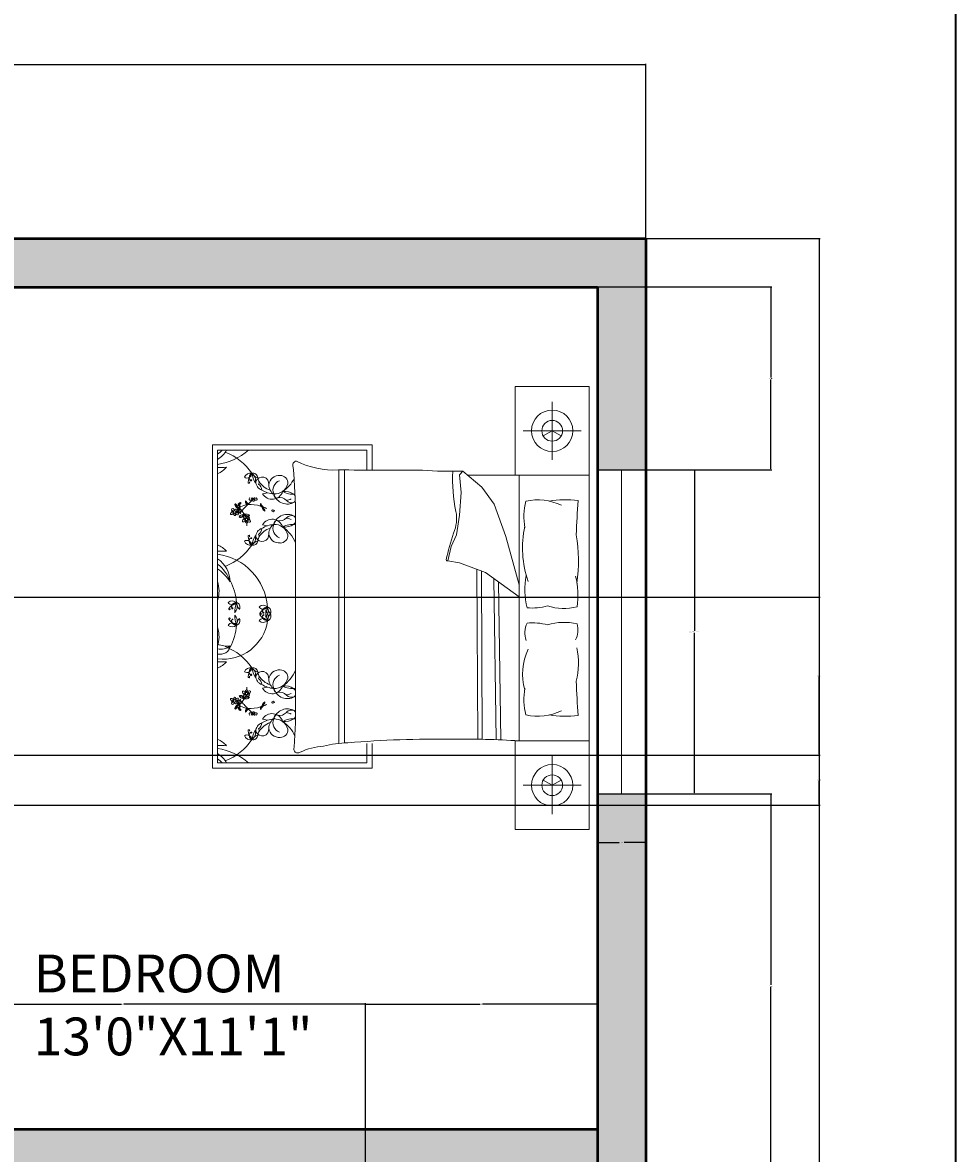
# Model space of a CAD drawing. Units: inches. Extents: x 1676 to 2199, y 1657 to 2783.
# Tile 9 of 10: x 2027 to 2199, y 2172 to 2381. Entities that reach past the tile are written whole.
import ezdxf

# ---------------------------------------------------------------- set-up
doc = ezdxf.new("R2010")
doc.units = ezdxf.units.IN
for name, color, linetype, lineweight in [('A-ANNO-DIMS', 2, 'Continuous', 18), ('A-ANNO-TTLB', 7, 'Continuous', 35), ('A-AREA-IDEN', 7, 'Continuous', 18), ('A-FURN', 8, 'Continuous', 13), ('A-GLAZ', 4, 'Continuous', 18), ('A-WALL', 7, 'Continuous', 50)]:
    doc.layers.add(name, color=color, linetype=linetype, lineweight=lineweight)
doc.layers.add('A-WALL-PATT', color=251, linetype='Continuous', lineweight=13, true_color=0x636466)
doc.styles.get("Standard").update_dxf_attribs({"font": 'arial.ttf'})
doc.dimstyles.get("Standard").update_dxf_attribs({"dimtxt": 0.18, "dimasz": 0.18, "dimexe": 0.18, "dimexo": 0.0625, "dimgap": 0.09, "dimtad": 0, "dimtih": 1, "dimtoh": 1, "dimdec": 4, "dimzin": 0, "dimdsep": 46, "dimtxsty": 'Standard', "dimcen": 0.09, "dimadec": 0, "dimazin": 0, "dimtfac": 1, "dimtdec": 4, "dimtofl": 0, "dimtmove": 0, "dimatfit": 3, "dimfxl": 1, "dimtolj": 1, "dimtzin": 0, "dimarcsym": 0})

# ---------------------------------------------------------------- blocks, each defined once
blk = doc.blocks.new('BED-DOUBLE-WITH-NIGHTSTANDS')
for p, q in [((0, 0), (0, -82.08)), ((-6.84, -13.57), (-6.84, -2.85)), ((-12.2, -8.21), (-1.48, -8.21)), ((-69.81, -10.83), (-40.24, -10.83)), ((-69.81, -70.68), (-69.81, -10.83)), ((-68.85, -11.79), (-68.85, -69.72)), ((-41.19, -11.79), (-68.85, -11.79)), ((-41.19, -15.48), (-41.19, -11.79)), ((-40.24, -10.83), (-40.24, -15.48)), ((-46.38, -66.12), (-46.38, -15.47)), ((-45.36, -66.04), (-45.36, -15.47)), ((-24.05, -16.35), (-23.39, -15.68)), ((-23.72, -19.67), (-24.05, -16.35)), ((-23.39, -15.68), (-19.9, -18.67)), ((0, -16.42), (-22.53, -16.42)), ((-12.97, -16.42), (-12.97, -65.67)), ((-19.9, -18.67), (-17.57, -21.83)), ((-60.53, -19.87), (-59.61, -19.69)), ((-24.05, -23.83), (-23.72, -19.67)), ((-17.57, -21.83), (-15.41, -27.82)), ((-54.44, -57.71), (-54.44, -24.38)), ((-24.55, -27.49), (-24.05, -23.83)), ((-60.53, -25.61), (-59.61, -25.79)), ((-25.55, -29.65), (-24.55, -27.49)), ((-15.41, -27.82), (-12.97, -36.77)), ((-26.21, -32.31), (-25.55, -29.65)), ((-24.05, -32.64), (-26.21, -32.31)), ((-19.23, -34.47), (-24.05, -32.64)), ((-20.65, -65.38), (-20.78, -33.88)), ((-19.81, -65.37), (-19.93, -34.2)), ((-12.97, -38.97), (-19.23, -34.47)), ((-17.22, -65.41), (-17.64, -35.61)), ((-16.38, -65.45), (-16.79, -36.22)), ((-60.53, -55.9), (-59.61, -55.72)), ((-60.53, -61.64), (-59.61, -61.82)), ((-41.19, -69.72), (-41.19, -66.11)), ((-40.24, -66.12), (-40.24, -70.68)), ((-6.84, -68.51), (-6.84, -79.24)), ((-40.24, -70.68), (-69.81, -70.68)), ((-68.85, -69.72), (-41.19, -69.72)), ((-12.2, -73.87), (-1.48, -73.87))]:
    blk.add_line(p, q)
for points in [[(-13.68, -16.42), (-13.68, 0), (0, 0)], [(-6.84, -8.21), (-8.5, -9.17)], [(-6.84, -8.21), (-5.18, -9.17)], [(0, -65.67), (-13.68, -65.67), (-13.68, -82.08), (0, -82.08)], [(-6.84, -73.87), (-8.5, -72.92)], [(-6.84, -73.87), (-5.18, -72.92)]]:
    blk.add_lwpolyline(points)
for points in [[(-30.9, -15.51, 0.001242), (-46.48, -15.47, -0.127202), (-54.24, -13.83)], [(-2.05, -21.13, 0.074897), (-7.41, -21.23, -0.472817)], [(-7.71, -40.66, 0.14099), (-2.24, -40.82, 0.235245)], [(-7.71, -44.16, -0.14099), (-2.24, -44, -0.235245)], [(-2.05, -60.95, -0.074897), (-7.41, -60.85, 0.472817)], [(-44.71, -66.02, 0.056112), (-49.23, -66.61, 0.095341), (-53.58, -67.77)]]:
    blk.add_lwpolyline(points, format="xyb")
for centre, radius in [((-6.84, -8.21), 3.83), ((-6.84, -8.21), 1.92), ((-65.71, -23.25), 0.209), ((-63.51, -24.62), 0.209), ((-65.71, -58.26), 0.209), ((-63.51, -56.89), 0.209), ((-6.84, -73.87), 3.83), ((-6.84, -73.87), 1.92)]:
    blk.add_circle(centre, radius)
for centre, radius, start, end in [((-72.71, -7.3), 6.51, 306.3036, 316.4814), ((-71.73, -9.18), 5.22, 303.4617, 330.1116), ((-70.3, -3.81), 10.72, 277.745, 311.8856), ((-71.36, -22.14), 10.72, 34.3865, 68.5908), ((-54.19, -14.58), 0.757, 93.98, 207.3412), ((-70.53, -12.11), 4.36, 292.5547, 318.9546), ((-68.18, -0.17), 14.83, 267.4081, 273.6519), ((-62.77, -17.25), 1.19, 77.7115, 159.0387), ((-63.41, -16.06), 0.895, 238.4633, 358.2869), ((-60.47, -17.87), 2.71, 138.8402, 177.9352), ((-62.11, -16.87), 0.877, 117.6827, 223.7762), ((-62.3, -16.95), 0.889, 2.9516, 103.728), ((-55.19, -14.46), 7.5, 192.5173, 207.1824), ((-63.5, -17.46), 1.69, 345.4653, 54.2343), ((-60.95, -15.14), 1.83, 211.3827, 255.2969), ((-57.44, -18.45), 1.96, 84.9449, 172.8857), ((-57.24, -17.88), 1.39, 354.4856, 91.0538), ((-139.89, -23.4), 85.45, 359.3433, 5.6887), ((-25.43, 59.58), 75.29, 265.8294, 271.553), ((5.68, -17.09), 30.98, 177.4519, 191.3392), ((-63.05, -17.78), 0.133, 177.9352, 11.4834), ((-62.98, -17.77), 0.0647, 11.4834, 127.9409), ((-62.66, -17.39), 0.116, 223.7762, 159.7183), ((-60.23, -17.7), 1.54, 175.969, 254.3045), ((-60.6, -18), 1.23, 350.264, 160.8688), ((-61.93, -17.74), 0.755, 333.9755, 53.2681), ((-62.27, -19.36), 1.64, 6.1662, 51.5825), ((-57.89, -15.55), 3.88, 211.2614, 251.7045), ((-57, -18.11), 2.38, 182.3591, 234.0401), ((-56.7, -19.22), 1.9, 111.5819, 201.4221), ((-58.27, -17.45), 2.47, 265.2933, 346.921), ((-60.22, -14.26), 6.21, 303.6671, 333.2997), ((-62.86, -20.88), 0.16, 142.4737, 265.053), ((-62.65, -20.85), 0.345, 127.7621, 169.0403), ((-62.84, -20.56), 0.486, 265.053, 338.3618), ((-62.19, -21.22), 0.635, 113.4276, 137.6104), ((-62.27, -20.56), 0.209, 183.2768, 356.7232), ((-62.11, -20.94), 0.342, 139.7889, 227.6792), ((-62.92, -20.94), 0.684, 353.0852, 15.7171), ((-62.47, -21.02), 0.432, 350.3487, 43.6538), ((-61.67, -20.57), 0.503, 198.7263, 262.5032), ((-62.07, -20.81), 0.2, 1.1081, 91.8675), ((-61.94, -20.85), 0.349, 11.5637, 52.6358), ((-61.69, -20.92), 0.162, 255.2356, 54.9248), ((-58.2, -15.52), 4.4, 236.2883, 266.5076), ((-58.76, -18.86), 2.04, 209.9085, 343.1337), ((-57.91, -20.15), 0.509, 167.3041, 285.1471), ((-56.53, -22.59), 3.17, 122.7011, 126.3445), ((-55.93, -19.17), 2.62, 199.2822, 299.1751), ((-57.33, -22.26), 1.68, 41.5653, 105.1471), ((-55.05, -16.54), 3.4, 238.8218, 279.1554), ((-56.53, -22.59), 3.17, 55.785, 94.7304), ((-56.41, -18.78), 2.36, 277.436, 299.9149), ((-55.35, -20.75), 0.989, 30.0293, 52.325), ((-65.87, -22.82), 0.413, 157.4086, 261.4386), ((-66.1, -22.81), 0.207, 58.0499, 135.6268), ((-65.89, -22.94), 0.138, 172.906, 277.132), ((-66.34, -23.19), 0.659, 14.7558, 58.0499), ((-65.42, -23.02), 0.285, 36.1046, 181.4281), ((-65.41, -21.9), 0.233, 124.3538, 214.3923), ((-65.06, -21.94), 0.544, 190.3057, 287.1958), ((-65.59, -22.79), 0.288, 270.0645, 331.1507), ((-64.91, -21.74), 0.632, 176.9701, 248.2913), ((-60.4, -18.41), 6.11, 212.6784, 216.3746), ((-65.34, -22.99), 0.205, 263.7526, 41.7054), ((-65.12, -21.89), 0.242, 216.3746, 291.7548), ((-62.98, -25.28), 3.41, 124.0033, 132.4917), ((-66.49, -25.71), 3.64, 63.7819, 68.2913), ((-64.54, -22.91), 0.579, 128.3208, 208.8162), ((-64.54, -22.06), 0.544, 122.8155, 187.3992), ((-64.96, -22.28), 0.182, 289.3605, 111.7548), ((-64.83, -22.28), 0.182, 221.8703, 44.2646), ((-64, -22.81), 0.953, 157.2305, 229.0635), ((-64.3, -22.13), 0.632, 109.4799, 177.6828), ((-64.32, -22.5), 0.561, 174.4544, 220.6188), ((-67.51, -25.63), 4.09, 30.544, 49.818), ((-64.64, -21.73), 0.233, 56.8636, 146.9021), ((-64.52, -21.99), 0.242, 148.8844, 224.2646), ((-65.26, -23.3), 0.674, 340.0041, 40.6188), ((-59.5, -25.02), 6.11, 145.1882, 148.8844), ((-62.98, -25.28), 3.41, 94.756, 119.2041), ((-55.72, -30.19), 11.22, 132.2412, 142.1744), ((-61.39, -21.26), 2.31, 178.3264, 187.1302), ((-63.89, -21.58), 0.431, 11.3256, 64.4621), ((-62.42, -20.96), 1.3, 190.2588, 210.656), ((-63.29, -21.49), 0.394, 188.3432, 274.2869), ((-62.95, -21.27), 0.688, 210.656, 242.6341), ((-62.43, -20.68), 1.32, 218.2101, 226.3071), ((-63.4, -21.79), 0.167, 325.7657, 67.4417), ((-68.6, -16.2), 7.79, 313.1541, 322.0459), ((-62.81, -28.67), 6.8, 73.5842, 93.8277), ((-62.22, -21.06), 0.18, 227.6792, 350.3487), ((-58.62, -21.75), 2.31, 178.3264, 187.1302), ((-61.12, -22.07), 0.431, 11.3256, 64.4621), ((-59.66, -21.45), 1.3, 190.2588, 210.656), ((-60.53, -21.98), 0.394, 188.3432, 274.2869), ((-60.19, -21.76), 0.688, 210.656, 242.6341), ((-59.67, -21.17), 1.32, 218.2101, 226.3071), ((-60.64, -22.28), 0.167, 325.7657, 67.4417), ((-60.17, -22.58), 0.394, 147.5332, 233.4768), ((-59.81, -22.38), 0.688, 179.1859, 211.164), ((-60.49, -22.54), 0.167, 354.3784, 96.0543), ((-62.81, -28.67), 6.8, 63.0032, 69.8941), ((-59.29, -22.07), 1.3, 211.164, 231.5612), ((-59.07, -21.01), 2.31, 234.6898, 243.4936), ((-59.05, -22.2), 1.32, 195.5129, 203.6099), ((-60.53, -23.06), 0.431, 357.3579, 50.4944), ((-58.68, -22.98), 0.158, 12.7051, 190.4384), ((-58.58, -22.96), 0.257, 190.4384, 10.4136), ((-55.16, -20.33), 1.23, 221.5653, 293.8354), ((-55.35, -20.75), 0.989, 314.4517, 333.558), ((-1.09, -24.06), 11, 165.1039, 191.0369), ((-9.56, -31.59), 10.58, 65.1316, 101.7583), ((779.11, -66.37), 782.47, 176.68521, 177.14978), ((-66.31, -23.57), 0.16, 142.4737, 265.053), ((-66.1, -23.53), 0.345, 61.2196, 169.0403), ((-66.28, -23.24), 0.486, 265.053, 338.3618), ((-65.64, -23.91), 0.635, 113.4276, 137.6104), ((-65.56, -23.63), 0.342, 139.7889, 227.6792), ((-65.67, -23.75), 0.18, 227.6792, 350.3487), ((-66.36, -23.62), 0.684, 353.0852, 15.7171), ((-65.91, -23.7), 0.432, 350.3487, 43.6538), ((-65.34, -22.86), 0.329, 221.8413, 265.7877), ((-65.11, -23.26), 0.503, 198.7263, 262.5032), ((-65.51, -23.49), 0.2, 1.1081, 91.8675), ((-65.39, -23.54), 0.349, 11.5637, 86.365), ((-65.14, -23.6), 0.162, 255.2356, 54.9248), ((-64.44, -22.87), 0.692, 207.7043, 254.3516), ((-64.89, -23.26), 0.953, 270.278, 342.111), ((-64.25, -24.45), 0.674, 98.7227, 159.3375), ((-64.59, -23.59), 0.692, 244.9899, 291.6373), ((-64.44, -23.23), 0.561, 278.7227, 324.8872), ((-64.54, -23.69), 0.579, 290.5253, 358.5375), ((-64.11, -24.93), 0.16, 142.4737, 265.053), ((-63.89, -24.9), 0.345, 61.2196, 169.0403), ((-64.08, -24.61), 0.486, 265.053, 338.3618), ((-63.67, -24.19), 0.413, 157.4086, 261.4386), ((-63.9, -24.18), 0.207, 58.0499, 135.6268), ((-63.41, -23.52), 0.579, 182.8499, 266.1226), ((-63.63, -23.12), 0.561, 231.7607, 277.9252), ((-63.2, -23.02), 0.953, 214.5369, 286.3699), ((-63.43, -25.27), 0.635, 113.4276, 137.6104), ((-63.68, -24.31), 0.138, 172.906, 277.132), ((-64.14, -24.56), 0.659, 14.7558, 58.0499), ((-67.51, -25.63), 4.09, 23.0501, 23.8477), ((-63.35, -24.99), 0.342, 139.7889, 227.6792), ((-63.46, -24.34), 0.674, 37.3105, 97.9252), ((-63.22, -24.39), 0.285, 36.1046, 181.4281), ((-64.16, -24.99), 0.684, 353.0852, 15.7171), ((-63.39, -23.41), 0.692, 265.0106, 311.658), ((-63.71, -25.07), 0.432, 350.3487, 43.6538), ((-62.91, -24.63), 0.503, 198.7263, 262.5032), ((-63.38, -24.16), 0.288, 270.0645, 331.1507), ((-63.14, -24.23), 0.329, 221.8413, 265.7877), ((-63.31, -24.86), 0.2, 1.1081, 91.8675), ((-63.14, -24.35), 0.205, 263.7526, 41.7054), ((-63.18, -24.91), 0.349, 11.5637, 86.365), ((-62.93, -24.97), 0.162, 255.2356, 54.9248), ((-58.76, -26.63), 2.04, 16.8663, 150.0915), ((-57.91, -25.34), 0.509, 74.8529, 192.6959), ((-55.93, -26.31), 2.62, 60.8249, 160.7178), ((-57.33, -23.22), 1.68, 254.8529, 318.4347), ((-56.41, -26.71), 2.36, 60.0851, 82.564), ((-55.16, -25.15), 1.23, 66.1646, 138.4347), ((-55.35, -24.73), 0.989, 307.675, 336.7144), ((-55.35, -24.73), 0.989, 23.229, 45.5483), ((-31.24, -24.49), 6.68, 336.2616, 11.3392), ((-63.46, -25.11), 0.18, 227.6792, 350.3487), ((-67.51, -25.63), 4.09, 357.1071, 4.7585), ((-60.23, -27.78), 1.54, 105.6955, 184.031), ((-62.27, -26.13), 1.64, 308.4175, 353.8338), ((-57.89, -29.93), 3.88, 108.2955, 148.7386), ((-58.2, -29.97), 4.4, 93.4924, 123.7117), ((-57, -27.38), 2.38, 125.9599, 177.6409), ((-56.7, -26.27), 1.9, 158.5779, 248.4181), ((-58.27, -28.03), 2.47, 13.079, 94.7067), ((-56.53, -22.9), 3.17, 233.6555, 237.2989), ((-55.05, -28.95), 3.4, 79.7133, 121.1782), ((-56.53, -22.9), 3.17, 265.2696, 304.215), ((-60.22, -31.22), 6.21, 21.4941, 56.3329), ((4.81, -38.01), 31.83, 160.1194, 169.3383), ((6.73, -29.85), 19.08, 168.0397, 199.2615), ((-63.41, -29.42), 0.895, 1.7131, 121.5367), ((-62.77, -28.23), 1.19, 200.9613, 282.2885), ((-63.05, -27.7), 0.133, 348.5166, 182.0648), ((-60.47, -27.61), 2.71, 182.0648, 221.1598), ((-62.98, -27.72), 0.0647, 232.0591, 348.5166), ((-62.11, -28.62), 0.877, 136.2238, 242.3173), ((-62.61, -28.1), 0.0699, 200.2667, 136.2271), ((-63.5, -28.02), 1.69, 305.7657, 14.5347), ((-55.19, -31.02), 7.5, 152.8176, 167.4827), ((-62.3, -28.53), 0.889, 256.272, 357.0484), ((-60.95, -30.35), 1.83, 104.7031, 148.6173), ((-60.6, -27.49), 1.23, 199.1312, 9.736), ((-61.93, -27.74), 0.755, 306.7319, 26.0245), ((-57.44, -27.04), 1.96, 187.1143, 275.0551), ((-57.24, -27.61), 1.39, 268.9462, 5.5144), ((-31.75, -32.38), 29.77, 352.2196, 9.497), ((-70.53, -33.38), 4.36, 41.0454, 67.4453), ((-68.18, -45.32), 14.83, 86.3481, 92.5919), ((-70.3, -41.68), 10.72, 4.4623, 82.255), ((-71.36, -23.34), 10.72, 291.4092, 325.6135), ((-71.73, -36.3), 5.22, 1.272, 56.5383), ((-72.71, -38.18), 6.51, 17.8504, 53.6964), ((-26.28, -32.12), 0.198, 178.8623, 289.7536), ((-74.54, -41.6), 9.68, 34.0123, 54.053), ((2.57, -37.57), 14.48, 169.8617, 193.6238), ((-16.7, -38.67), 14.63, 351.5249, 13.96), ((-74.49, -37.86), 5.89, 343.5431, 17.0202), ((-76.04, -40.86), 10.72, 4.4623, 27.4146), ((-77.53, -40.2), 8.72, 4.3787, 5.6357), ((-83.5, -44.79), 15.58, 19.7217, 19.9028), ((-66.15, -40.91), 1.19, 47.7873, 129.1145), ((-66.12, -39.56), 0.895, 208.5391, 328.3627), ((-66.66, -41.22), 0.133, 148.011, 341.5592), ((-64.48, -42.59), 2.71, 108.9159, 148.011), ((-66.6, -41.25), 0.0647, 341.5592, 98.0167), ((-65.39, -40.9), 0.877, 87.7585, 193.852), ((-66.13, -41.08), 0.116, 193.852, 129.9245), ((-58.2, -42.27), 7.5, 162.593, 177.2582), ((-66.9, -40.72), 1.69, 315.5411, 24.3101), ((-63.52, -39.98), 1.83, 181.4585, 225.3727), ((-65.6, -40.88), 0.889, 333.0274, 73.8037), ((-60.41, -41.73), 1.19, 47.7873, 129.1145), ((-60.38, -40.38), 0.895, 208.5391, 328.3627), ((-58.73, -43.41), 2.71, 108.9159, 148.011), ((-59.65, -41.72), 0.877, 87.7585, 193.852), ((-60.39, -41.9), 0.116, 193.852, 129.9245), ((-61.16, -41.54), 1.69, 315.5411, 24.3101), ((-52.46, -43.09), 7.5, 162.593, 177.2582), ((-61.16, -42.7), 1.69, 335.6899, 44.4589), ((-52.46, -41.16), 7.5, 182.7418, 197.407), ((-59.86, -41.7), 0.889, 333.0274, 73.8037), ((-57.78, -40.8), 1.83, 181.4585, 225.3727), ((-10.45, -30.98), 10.06, 264.0129, 285.8293), ((-67.82, -42.22), 8.3, 262.8636, 351.8197), ((-66.12, -44.69), 0.895, 31.6373, 151.4609), ((-66.66, -43.02), 0.133, 18.4408, 211.989), ((-64.48, -41.66), 2.71, 211.989, 251.0841), ((-66.6, -43), 0.0647, 261.9833, 18.4408), ((-65.39, -43.35), 0.877, 166.148, 272.2415), ((-66.08, -43.15), 0.0699, 230.1909, 166.0209), ((-58.2, -41.98), 7.5, 182.7418, 197.407), ((-66.9, -43.52), 1.69, 335.6899, 44.4589), ((-63.52, -44.27), 1.83, 134.6273, 178.5415), ((-65.6, -43.37), 0.889, 286.1963, 26.9726), ((-60.38, -43.87), 0.895, 31.6373, 151.4609), ((-60.41, -42.52), 1.19, 230.8855, 312.2127), ((-60.92, -42.04), 0.133, 148.011, 341.5592), ((-60.92, -42.2), 0.133, 18.4408, 211.989), ((-58.73, -40.84), 2.71, 211.989, 251.0841), ((-60.86, -42.07), 0.0647, 341.5592, 98.0167), ((-60.86, -42.18), 0.0647, 261.9833, 18.4408), ((-59.65, -42.52), 0.877, 166.148, 272.2415), ((-60.34, -42.33), 0.0699, 230.1909, 166.0209), ((-59.86, -42.55), 0.889, 286.1963, 26.9726), ((-57.78, -43.45), 1.83, 134.6273, 178.5415), ((-7.56, -45.67), 4.35, 155.0183, 198.5407), ((-10.45, -53.84), 10.06, 74.1707, 95.9871), ((-74.49, -46.39), 5.89, 342.9798, 16.4569), ((-77.53, -44.05), 8.72, 354.3643, 355.6213), ((-83.5, -39.46), 15.58, 340.0972, 340.2783), ((-66.15, -43.34), 1.19, 230.8855, 312.2127), ((-76.04, -43.39), 10.72, 332.5854, 355.5377), ((-6.14, -45.12), 4.06, 333.3437, 16.1026), ((-67.07, -43.29), 4.8, 248.117, 276.6195), ((-68.4, -47.7), 1.92, 256.3898, 349.0739), ((-68.14, -46.25), 2.43, 252.8609, 311.9049), ((-71.36, -58.17), 10.72, 34.3865, 68.5908), ((-1.9, -53.28), 10.45, 153.8761, 196.1746), ((-16.41, -51.21), 14.43, 346.3427, 11.1841), ((-68.18, -36.19), 14.83, 267.4081, 273.6519), ((-70.53, -48.13), 4.36, 292.5547, 318.9546), ((-62.77, -53.28), 1.19, 77.7115, 159.0387), ((-63.41, -52.09), 0.895, 238.4633, 358.2869), ((-60.47, -53.9), 2.71, 138.8402, 177.9352), ((-62.11, -52.89), 0.877, 117.6827, 223.7762), ((-62.3, -52.98), 0.889, 2.9516, 103.728), ((-60.95, -51.16), 1.83, 211.3827, 255.2969), ((-63.5, -53.49), 1.69, 345.4653, 54.2343), ((-55.19, -50.49), 7.5, 192.5173, 207.1824), ((-63.05, -53.81), 0.133, 177.9352, 11.4834), ((-62.98, -53.79), 0.0647, 11.4834, 127.9409), ((-62.66, -53.42), 0.116, 223.7762, 159.7183), ((-60.23, -53.73), 1.54, 175.969, 254.3045), ((-60.6, -54.02), 1.23, 350.264, 160.8688), ((-61.93, -53.77), 0.755, 333.9755, 53.2681), ((-62.27, -55.38), 1.64, 6.1662, 51.5825), ((-57.89, -51.58), 3.88, 211.2614, 251.7045), ((-57.44, -54.47), 1.96, 84.9449, 172.8857), ((-57, -54.13), 2.38, 182.3591, 234.0401), ((-56.7, -55.24), 1.9, 111.5819, 201.4221), ((-58.27, -53.48), 2.47, 265.2933, 346.921), ((-57.24, -53.9), 1.39, 354.4856, 91.0538), ((-60.22, -50.29), 6.21, 303.6671, 338.5059), ((-64.11, -56.58), 0.16, 94.947, 217.5263), ((-64.08, -56.9), 0.486, 21.6382, 94.947), ((-63.35, -56.52), 0.342, 132.3208, 220.2111), ((-63.46, -56.4), 0.18, 9.6513, 132.3208), ((-64.16, -56.52), 0.684, 344.2829, 6.9148), ((-67.51, -55.88), 4.09, 355.2415, 2.8929), ((-63.71, -56.44), 0.432, 316.3462, 9.6513), ((-62.91, -56.88), 0.503, 97.4968, 161.2737), ((-62.93, -56.54), 0.162, 305.0752, 104.7644), ((-58.2, -51.54), 4.4, 236.2883, 266.5076), ((-58.76, -54.88), 2.04, 209.9085, 343.1337), ((-57.91, -56.17), 0.509, 167.3041, 285.1471), ((-56.53, -58.61), 3.17, 122.7011, 126.3445), ((-55.93, -55.2), 2.62, 199.2822, 299.1751), ((-55.05, -52.56), 3.4, 238.8218, 280.2867), ((-56.53, -58.61), 3.17, 55.785, 94.7304), ((-55.35, -56.78), 0.989, 23.2856, 52.325), ((-1.09, -58.02), 11, 168.9631, 194.8961), ((779.11, -15.71), 782.47, 182.85022, 183.31479), ((-66.31, -57.94), 0.16, 94.947, 217.5263), ((-66.1, -57.98), 0.345, 190.9597, 298.7804), ((-66.28, -58.27), 0.486, 21.6382, 94.947), ((-65.87, -58.69), 0.413, 98.5614, 202.5914), ((-65.64, -57.6), 0.635, 222.3896, 246.5724), ((-65.89, -58.57), 0.138, 82.868, 187.094), ((-66.34, -58.32), 0.659, 301.9501, 345.2442), ((-65.56, -57.88), 0.342, 132.3208, 220.2111), ((-65.67, -57.76), 0.18, 9.6513, 132.3208), ((-66.36, -57.89), 0.684, 344.2829, 6.9148), ((-65.42, -58.49), 0.285, 178.5719, 323.8954), ((-65.91, -57.81), 0.432, 316.3462, 9.6513), ((-65.11, -58.25), 0.503, 97.4968, 161.2737), ((-65.34, -58.65), 0.329, 94.2123, 138.1587), ((-65.59, -58.72), 0.288, 28.8493, 89.9355), ((-65.51, -58.02), 0.2, 268.1325, 358.8919), ((-65.39, -57.97), 0.349, 273.635, 348.4363), ((-65.34, -58.52), 0.205, 318.2946, 96.2474), ((-65.14, -57.91), 0.162, 305.0752, 104.7644), ((-64.54, -58.6), 0.579, 151.1838, 231.6792), ((-64.44, -58.64), 0.692, 105.6484, 152.2957), ((-64, -58.7), 0.953, 130.9365, 202.7695), ((-64.59, -57.92), 0.692, 68.3627, 115.0101), ((-64.89, -58.25), 0.953, 17.889, 89.722), ((-64.25, -57.06), 0.674, 200.6625, 261.2773), ((-64.32, -59.01), 0.561, 139.3812, 185.5456), ((-67.51, -55.88), 4.09, 310.182, 329.456), ((-65.26, -58.21), 0.674, 319.3812, 19.9959), ((-55.72, -51.32), 11.22, 217.8256, 227.7588), ((-64.44, -58.28), 0.561, 35.1128, 81.2773), ((-64.54, -57.82), 0.579, 1.4625, 69.4747), ((-63.89, -56.61), 0.345, 190.9597, 298.7804), ((-63.67, -57.32), 0.413, 98.5614, 202.5914), ((-63.9, -57.33), 0.207, 224.3732, 301.9501), ((-63.41, -57.99), 0.579, 93.8774, 177.1501), ((-63.2, -58.49), 0.953, 73.6301, 145.4631), ((-63.63, -58.39), 0.561, 82.0748, 128.2393), ((-63.43, -56.24), 0.635, 222.3896, 246.5724), ((-63.68, -57.2), 0.138, 82.868, 187.094), ((-64.14, -56.95), 0.659, 301.9501, 345.2442), ((-67.51, -55.88), 4.09, 336.1523, 336.9499), ((-63.46, -57.17), 0.674, 262.0748, 322.6895), ((-63.22, -57.12), 0.285, 178.5719, 323.8954), ((-63.39, -58.1), 0.692, 48.342, 94.9894), ((-63.14, -57.28), 0.329, 94.2123, 138.1587), ((-63.38, -57.35), 0.288, 28.8493, 89.9355), ((-63.31, -56.65), 0.2, 268.1325, 358.8919), ((-63.18, -56.6), 0.349, 273.635, 348.4363), ((-63.14, -57.16), 0.205, 318.2946, 96.2474), ((-60.17, -58.93), 0.394, 126.5232, 212.4668), ((-59.29, -59.44), 1.3, 128.4388, 148.836), ((-59.07, -60.5), 2.31, 116.5064, 125.3102), ((-60.53, -58.45), 0.431, 309.5056, 2.6421), ((-58.68, -58.53), 0.158, 169.5616, 347.2949), ((-58.58, -58.55), 0.257, 349.5864, 169.5616), ((-57.33, -58.29), 1.68, 41.5653, 105.1471), ((-56.41, -54.8), 2.36, 277.436, 299.9149), ((-55.16, -56.36), 1.23, 221.5653, 293.8354), ((-134.28, -60.22), 79.87, 355.2402, 1.8035), ((-55.35, -56.78), 0.989, 314.4517, 336.7144), ((-66.1, -58.7), 0.207, 224.3732, 301.9501), ((-65.41, -59.61), 0.233, 145.6077, 235.6462), ((-65.06, -59.58), 0.544, 72.8042, 169.6943), ((-64.91, -59.77), 0.632, 111.7087, 183.0299), ((-60.4, -63.1), 6.11, 143.6254, 147.3216), ((-65.12, -59.62), 0.242, 68.2452, 143.6254), ((-62.98, -56.23), 3.41, 227.5083, 235.9967), ((-66.49, -55.8), 3.64, 291.7087, 296.2181), ((-64.54, -59.45), 0.544, 172.6008, 237.1845), ((-64.96, -59.23), 0.182, 248.2452, 70.6395), ((-64.83, -59.23), 0.182, 315.7354, 138.1297), ((-64.3, -59.38), 0.632, 182.3172, 250.5201), ((-64.64, -59.78), 0.233, 213.0979, 303.1364), ((-64.52, -59.52), 0.242, 135.7354, 211.1156), ((-59.5, -56.49), 6.11, 211.1156, 214.8118), ((-62.98, -56.23), 3.41, 240.7959, 265.244), ((-62.42, -60.55), 1.3, 149.344, 169.7412), ((-61.39, -60.25), 2.31, 172.8698, 181.6736), ((-63.89, -59.93), 0.431, 295.5379, 348.6744), ((-63.29, -60.02), 0.394, 85.7131, 171.6568), ((-62.95, -60.24), 0.688, 117.3659, 149.344), ((-62.43, -60.83), 1.32, 133.6929, 141.7899), ((-63.4, -59.72), 0.167, 292.5583, 34.2343), ((-62.81, -52.84), 6.8, 266.1723, 286.4158), ((-68.6, -65.31), 7.79, 37.9541, 46.8459), ((-62.86, -60.63), 0.16, 94.947, 217.5263), ((-62.65, -60.66), 0.345, 190.9597, 232.2379), ((-62.84, -60.95), 0.486, 21.6382, 94.947), ((-62.19, -60.29), 0.635, 222.3896, 246.5724), ((-62.27, -60.95), 0.209, 3.2768, 176.7232), ((-62.11, -60.57), 0.342, 132.3208, 220.2111), ((-62.22, -60.45), 0.18, 9.6513, 132.3208), ((-62.92, -60.57), 0.684, 344.2829, 6.9148), ((-62.47, -60.49), 0.432, 316.3462, 9.6513), ((-61.67, -60.94), 0.503, 97.4968, 161.2737), ((-62.07, -60.7), 0.2, 268.1325, 358.8919), ((-61.69, -60.6), 0.162, 305.0752, 104.7644), ((-61.94, -60.66), 0.349, 307.3642, 348.4363), ((-59.66, -60.06), 1.3, 149.344, 169.7412), ((-58.62, -59.76), 2.31, 172.8698, 181.6736), ((-61.12, -59.44), 0.431, 295.5379, 348.6744), ((-60.53, -59.53), 0.394, 85.7131, 171.6568), ((-60.19, -59.75), 0.688, 117.3659, 149.344), ((-59.67, -60.34), 1.32, 133.6929, 141.7899), ((-60.64, -59.23), 0.167, 292.5583, 34.2343), ((-58.76, -62.65), 2.04, 16.8663, 150.0915), ((-59.81, -59.13), 0.688, 148.836, 180.8141), ((-60.49, -58.97), 0.167, 263.9457, 5.6216), ((-62.81, -52.84), 6.8, 290.1059, 296.9968), ((-59.05, -59.31), 1.32, 156.3901, 164.4871), ((-55.93, -62.34), 2.62, 60.8249, 160.7178), ((-57.33, -59.25), 1.68, 254.8529, 318.4347), ((-56.41, -62.73), 2.36, 60.0851, 82.564), ((-55.16, -61.18), 1.23, 66.1646, 138.4347), ((-55.35, -60.76), 0.989, 16.6343, 45.5483), ((-9.56, -50.49), 10.58, 258.2417, 294.8684), ((-60.23, -63.81), 1.54, 105.6955, 184.031), ((-62.27, -62.15), 1.64, 308.4175, 353.8338), ((-57.89, -65.96), 3.88, 108.2955, 148.7386), ((-58.2, -65.99), 4.4, 93.4924, 123.7117), ((-57, -63.4), 2.38, 125.9599, 177.6409), ((-56.7, -62.29), 1.9, 158.5779, 248.4181), ((-58.27, -64.06), 2.47, 13.079, 94.7067), ((-57.91, -61.36), 0.509, 74.8529, 192.6959), ((-56.53, -58.92), 3.17, 233.6555, 237.2989), ((-55.05, -64.97), 3.4, 79.249, 121.1782), ((-56.53, -58.92), 3.17, 265.2696, 304.215), ((-60.22, -67.25), 6.21, 23.6453, 56.3329), ((-55.35, -60.76), 0.989, 307.675, 342.5814), ((-63.41, -65.45), 0.895, 1.7131, 121.5367), ((-62.77, -64.26), 1.19, 200.9613, 282.2885), ((-63.05, -63.73), 0.133, 348.5166, 182.0648), ((-60.47, -63.64), 2.71, 182.0648, 221.1598), ((-62.98, -63.74), 0.0647, 232.0591, 348.5166), ((-62.11, -64.64), 0.877, 136.2238, 242.3173), ((-62.61, -64.13), 0.0699, 200.2667, 136.2271), ((-55.19, -67.05), 7.5, 152.8176, 167.4827), ((-63.5, -64.05), 1.69, 305.7657, 14.5347), ((-60.95, -66.37), 1.83, 104.7031, 148.6173), ((-62.3, -64.56), 0.889, 256.272, 357.0484), ((-60.6, -63.51), 1.23, 199.1312, 9.736), ((-61.93, -63.77), 0.755, 306.7319, 26.0245), ((-57.44, -63.06), 1.96, 187.1143, 275.0551), ((-57.24, -63.63), 1.39, 268.9462, 5.5144), ((-70.53, -69.4), 4.36, 41.0454, 67.4453), ((-68.18, -81.34), 14.83, 86.3481, 92.5919), ((-71.36, -59.37), 10.72, 291.4092, 325.6135), ((-53.99, -67.14), 0.748, 156.5219, 303.8264), ((-28.37, -257.71), 192.39, 89.1145, 94.8735), ((-23, -212.81), 147.49, 86.1, 90.9282), ((-70.3, -77.7), 10.72, 48.1144, 82.255), ((-71.73, -72.33), 5.22, 29.8884, 56.5383), ((-72.71, -74.21), 6.51, 43.5186, 53.6964)]:
    blk.add_arc(centre, radius, start, end)
blk = doc.blocks.new('WIN-60')
for p, q in [((0, 0), (9, 0)), ((9, 0), (4.5, 0)), ((4.5, 0), (4.5, -60)), ((4.5, -60), (0, -60)), ((0, -60), (9, -60))]:
    blk.add_line(p, q)
blk = doc.blocks.new('*D7')
at = {"layer": 'A-ANNO-DIMS', "color": 0, "lineweight": -2, "transparency": 16777216}
for p, q in [((2142.14, 2298.21), (2151.25, 2298.21)), ((2151.07, 2298.03), (2151.07, 2268.39)), ((2151.07, 2238.39), (2151.07, 2268.03)), ((2142.14, 2238.21), (2151.25, 2238.21))]:
    blk.add_line(p, q, dxfattribs=at)
at = {"layer": 'A-ANNO-DIMS', "color": 0, "transparency": 16777216}
for points in [[(2151.04, 2298.03), (2151.1, 2298.03), (2151.07, 2298.21)], [(2151.04, 2238.39), (2151.1, 2238.39), (2151.07, 2238.21)]]:
    blk.add_solid(points, dxfattribs=at)
at = {"layer": 'Defpoints', "color": 0, "transparency": 16777216}
for p in [(2142.07, 2298.21), (2151.07, 2298.21), (2142.07, 2238.21)]:
    blk.add_point(p, dxfattribs=at)
at = {"layer": 'A-ANNO-DIMS', "color": 0, "transparency": 16777216, "insert": (2151.07, 2268.21), "char_height": 0.18, "attachment_point": 5}
blk.add_mtext('\\A1;WINDOW 60 TYP.', dxfattribs=at)
blk = doc.blocks.new('*D8')
at = {"layer": 'A-ANNO-DIMS', "color": 0, "lineweight": -2, "transparency": 16777216}
for p, q in [((2133.07, 2238.15), (2133.07, 2229.03)), ((2142.07, 2238.15), (2142.07, 2229.03)), ((2133.25, 2229.21), (2137.12, 2229.21)), ((2141.89, 2229.21), (2138.03, 2229.21))]:
    blk.add_line(p, q, dxfattribs=at)
at = {"layer": 'A-ANNO-DIMS', "color": 0, "transparency": 16777216}
for points in [[(2133.25, 2229.24), (2133.25, 2229.18), (2133.07, 2229.21)], [(2141.89, 2229.24), (2141.89, 2229.18), (2142.07, 2229.21)]]:
    blk.add_solid(points, dxfattribs=at)
at = {"layer": 'Defpoints', "color": 0, "transparency": 16777216}
for p in [(2133.07, 2238.21), (2142.07, 2238.21), (2142.07, 2229.21)]:
    blk.add_point(p, dxfattribs=at)
at = {"layer": 'A-ANNO-DIMS', "color": 0, "transparency": 16777216, "insert": (2137.57, 2229.21), "char_height": 0.18, "attachment_point": 5}
blk.add_mtext('\\A1;9 TYP.', dxfattribs=at)
blk = doc.blocks.new('*D19')
at = {"layer": 'A-ANNO-DIMS', "color": 0, "lineweight": -2, "transparency": 16777216}
for p, q in [((1755.07, 2341.15), (1755.07, 2373.42)), ((1755.25, 2373.24), (1948.29, 2373.24)), ((2141.89, 2373.24), (1948.86, 2373.24)), ((2142.07, 2341.15), (2142.07, 2373.42))]:
    blk.add_line(p, q, dxfattribs=at)
at = {"layer": 'A-ANNO-DIMS', "color": 0, "transparency": 16777216}
for points in [[(1755.25, 2373.27), (1755.25, 2373.21), (1755.07, 2373.24)], [(2141.89, 2373.27), (2141.89, 2373.21), (2142.07, 2373.24)]]:
    blk.add_solid(points, dxfattribs=at)
at = {"layer": 'Defpoints', "color": 0, "transparency": 16777216}
for p in [(2142.07, 2373.24), (1755.07, 2341.09), (2142.07, 2341.09)]:
    blk.add_point(p, dxfattribs=at)
at = {"layer": 'A-ANNO-DIMS', "color": 0, "transparency": 16777216, "insert": (1948.57, 2373.24), "char_height": 0.18, "attachment_point": 5}
blk.add_mtext('\\A1;387', dxfattribs=at)
blk = doc.blocks.new('*D20')
at = {"layer": 'A-ANNO-DIMS', "color": 0, "lineweight": -2, "transparency": 16777216}
for p, q in [((2142.14, 2341.09), (2174.4, 2341.09)), ((2174.22, 2340.91), (2174.22, 2061.27)), ((2174.22, 1781.27), (2174.22, 2060.91)), ((2142.14, 1781.09), (2174.4, 1781.09))]:
    blk.add_line(p, q, dxfattribs=at)
at = {"layer": 'A-ANNO-DIMS', "color": 0, "transparency": 16777216}
for points in [[(2174.19, 2340.91), (2174.25, 2340.91), (2174.22, 2341.09)], [(2174.19, 1781.27), (2174.25, 1781.27), (2174.22, 1781.09)]]:
    blk.add_solid(points, dxfattribs=at)
at = {"layer": 'Defpoints', "color": 0, "transparency": 16777216}
for p in [(2142.07, 2341.09), (2174.22, 2341.09), (2142.07, 1781.09)]:
    blk.add_point(p, dxfattribs=at)
at = {"layer": 'A-ANNO-DIMS', "color": 0, "transparency": 16777216, "insert": (2174.22, 2061.09), "char_height": 0.18, "attachment_point": 5}
blk.add_mtext('\\A1;560', dxfattribs=at)
blk = doc.blocks.new('*D35')
at = {"layer": 'A-ANNO-DIMS', "color": 0, "lineweight": -2, "transparency": 16777216}
for p, q in [((2133.14, 2238.21), (2165.4, 2238.21)), ((2165.22, 2238.03), (2165.22, 2202.83)), ((2165.22, 2167.27), (2165.22, 2202.47)), ((2133.14, 2167.09), (2165.4, 2167.09))]:
    blk.add_line(p, q, dxfattribs=at)
at = {"layer": 'A-ANNO-DIMS', "color": 0, "transparency": 16777216}
for points in [[(2165.19, 2238.03), (2165.25, 2238.03), (2165.22, 2238.21)], [(2165.19, 2167.27), (2165.25, 2167.27), (2165.22, 2167.09)]]:
    blk.add_solid(points, dxfattribs=at)
at = {"layer": 'Defpoints', "color": 0, "transparency": 16777216}
for p in [(2133.07, 2238.21), (2133.07, 2167.09), (2165.22, 2167.09)]:
    blk.add_point(p, dxfattribs=at)
at = {"layer": 'A-ANNO-DIMS', "color": 0, "transparency": 16777216, "insert": (2165.22, 2202.65), "char_height": 0.18, "attachment_point": 5}
blk.add_mtext('\\A1;71.12', dxfattribs=at)
blk = doc.blocks.new('*D36')
at = {"layer": 'A-ANNO-DIMS', "color": 0, "lineweight": -2, "transparency": 16777216}
for p, q in [((2133.14, 2332.09), (2165.4, 2332.09)), ((2165.22, 2331.91), (2165.22, 2315.33)), ((2165.22, 2298.39), (2165.22, 2314.97)), ((2133.14, 2298.21), (2165.4, 2298.21))]:
    blk.add_line(p, q, dxfattribs=at)
at = {"layer": 'A-ANNO-DIMS', "color": 0, "transparency": 16777216}
for points in [[(2165.19, 2331.91), (2165.25, 2331.91), (2165.22, 2332.09)], [(2165.19, 2298.39), (2165.25, 2298.39), (2165.22, 2298.21)]]:
    blk.add_solid(points, dxfattribs=at)
at = {"layer": 'Defpoints', "color": 0, "transparency": 16777216}
for p in [(2133.07, 2332.09), (2133.07, 2298.21), (2165.22, 2298.21)]:
    blk.add_point(p, dxfattribs=at)
at = {"layer": 'A-ANNO-DIMS', "color": 0, "transparency": 16777216, "insert": (2165.22, 2315.15), "char_height": 0.18, "attachment_point": 5}
blk.add_mtext('\\A1;33.88', dxfattribs=at)
blk = doc.blocks.new('*D41')
at = {"layer": 'A-ANNO-DIMS', "color": 0, "lineweight": -2, "transparency": 16777216}
for p, q in [((1991.14, 2245.34), (2174.4, 2245.34)), ((2174.22, 2245.16), (2174.22, 2240.9)), ((2174.22, 2236.27), (2174.22, 2240.53)), ((1991.14, 2236.09), (2174.4, 2236.09))]:
    blk.add_line(p, q, dxfattribs=at)
at = {"layer": 'A-ANNO-DIMS', "color": 0, "transparency": 16777216}
for points in [[(2174.19, 2245.16), (2174.25, 2245.16), (2174.22, 2245.34)], [(2174.19, 2236.27), (2174.25, 2236.27), (2174.22, 2236.09)]]:
    blk.add_solid(points, dxfattribs=at)
at = {"layer": 'Defpoints', "color": 0, "transparency": 16777216}
for p in [(1991.07, 2245.34), (2174.22, 2245.34), (1991.07, 2236.09)]:
    blk.add_point(p, dxfattribs=at)
at = {"layer": 'A-ANNO-DIMS', "color": 0, "transparency": 16777216, "insert": (2174.22, 2240.71), "char_height": 0.18, "attachment_point": 5}
blk.add_mtext('\\A1;9.255', dxfattribs=at)
blk = doc.blocks.new('*D42')
at = {"layer": 'A-ANNO-DIMS', "color": 0, "lineweight": -2, "transparency": 16777216}
for p, q in [((1991.14, 2274.63), (2174.4, 2274.63)), ((2174.22, 2274.45), (2174.22, 2260.17)), ((2174.22, 2245.52), (2174.22, 2259.81)), ((1991.14, 2245.34), (2174.4, 2245.34))]:
    blk.add_line(p, q, dxfattribs=at)
at = {"layer": 'A-ANNO-DIMS', "color": 0, "transparency": 16777216}
for points in [[(2174.19, 2274.45), (2174.25, 2274.45), (2174.22, 2274.63)], [(2174.19, 2245.52), (2174.25, 2245.52), (2174.22, 2245.34)]]:
    blk.add_solid(points, dxfattribs=at)
at = {"layer": 'Defpoints', "color": 0, "transparency": 16777216}
for p in [(1991.07, 2274.63), (2174.22, 2274.63), (1991.07, 2245.34)]:
    blk.add_point(p, dxfattribs=at)
at = {"layer": 'A-ANNO-DIMS', "color": 0, "transparency": 16777216, "insert": (2174.22, 2259.99), "char_height": 0.18, "attachment_point": 5}
blk.add_mtext('\\A1;29.29', dxfattribs=at)
blk = doc.blocks.new('*D45')
at = {"layer": 'A-ANNO-DIMS', "color": 0, "lineweight": -2, "transparency": 16777216}
for p, q in [((2000.07, 2167.15), (2000.07, 2199.42)), ((2000.25, 2199.24), (2044.86, 2199.24)), ((2089.89, 2199.24), (2045.29, 2199.24)), ((2090.07, 2167.15), (2090.07, 2199.42))]:
    blk.add_line(p, q, dxfattribs=at)
at = {"layer": 'A-ANNO-DIMS', "color": 0, "transparency": 16777216}
for points in [[(2000.25, 2199.27), (2000.25, 2199.21), (2000.07, 2199.24)], [(2089.89, 2199.27), (2089.89, 2199.21), (2090.07, 2199.24)]]:
    blk.add_solid(points, dxfattribs=at)
at = {"layer": 'Defpoints', "color": 0, "transparency": 16777216}
for p in [(2090.07, 2199.24), (2000.07, 2167.09), (2090.07, 2167.09)]:
    blk.add_point(p, dxfattribs=at)
at = {"layer": 'A-ANNO-DIMS', "color": 0, "transparency": 16777216, "insert": (2045.07, 2199.24), "char_height": 0.18, "attachment_point": 5}
blk.add_mtext('\\A1;90', dxfattribs=at)
blk = doc.blocks.new('*D46')
at = {"layer": 'A-ANNO-DIMS', "color": 0, "lineweight": -2, "transparency": 16777216}
for p, q in [((2090.07, 2167.15), (2090.07, 2199.42)), ((2090.25, 2199.24), (2111.35, 2199.24)), ((2132.89, 2199.24), (2111.8, 2199.24)), ((2133.07, 2167.15), (2133.07, 2199.42))]:
    blk.add_line(p, q, dxfattribs=at)
at = {"layer": 'A-ANNO-DIMS', "color": 0, "transparency": 16777216}
for points in [[(2090.25, 2199.27), (2090.25, 2199.21), (2090.07, 2199.24)], [(2132.89, 2199.27), (2132.89, 2199.21), (2133.07, 2199.24)]]:
    blk.add_solid(points, dxfattribs=at)
at = {"layer": 'Defpoints', "color": 0, "transparency": 16777216}
for p in [(2133.07, 2199.24), (2090.07, 2167.09), (2133.07, 2167.09)]:
    blk.add_point(p, dxfattribs=at)
at = {"layer": 'A-ANNO-DIMS', "color": 0, "transparency": 16777216, "insert": (2111.57, 2199.24), "char_height": 0.18, "attachment_point": 5}
blk.add_mtext('\\A1;43', dxfattribs=at)

msp = doc.modelspace()

# ---------------------------------------------------------------- hatches: boundary and pattern name
at = {"layer": 'A-WALL-PATT'}
h = msp.add_hatch(color=256, dxfattribs=at)
h.dxf.hatch_style = 1
h.paths.add_polyline_path([(1945.4216, 2336.5871), (1945.4216, 2341.0871), (1755.075, 2341.0871), (1755.075, 2323.0739), (1764.075, 2323.0739), (1764.075, 2332.0871), (1945.4216, 2332.0871)])
h.paths.add_polyline_path([(1764.075, 2299.0739), (1755.075, 2299.0739), (1755.075, 2266.2601), (1759.575, 2266.2601), (1764.075, 2266.2601)])
h.paths.add_polyline_path([(1843.075, 2285.0871), (1764.075, 2285.0871), (1764.075, 2276.0871), (1843.075, 2276.0871)])
h.paths.add_polyline_path([(1931.075, 2332.0871), (1922.075, 2332.0871), (1922.075, 2285.0871), (1907.247, 2285.0871), (1907.247, 2276.0871), (1922.075, 2276.0871), (1922.075, 2263.0871), (1922.075, 2214.434), (1922.075, 2183.2198), (1931.075, 2183.2198), (1931.075, 2214.434), (1931.075, 2227.0871), (1991.075, 2227.0871), (1991.075, 2176.0871), (1991.075, 2167.0871), (2000.075, 2167.0871), (2133.075, 2167.0871), (2133.075, 2176.0871), (2000.075, 2176.0871), (2000.075, 2245.3418), (1995.575, 2245.3418), (1991.075, 2245.3418), (1991.075, 2236.0871), (1931.075, 2236.0871)])
h.paths.add_polyline_path([(2000.075, 2332.0871), (1991.075, 2332.0871), (1991.075, 2285.0871), (1991.075, 2274.6339), (2000.075, 2274.6339), (2000.075, 2285.0871)], flags=17)
h.paths.add_polyline_path([(2142.075, 2341.0871), (1969.4216, 2341.0871), (1969.4216, 2332.0871), (2133.075, 2332.0871), (2133.075, 2298.2101), (2142.075, 2298.2101)])
h.paths.add_polyline_path([(2142.075, 1844.9908), (2133.075, 1844.9908), (2133.075, 1790.0871), (2061.2106, 1790.0871), (2061.2106, 1781.0871), (2142.075, 1781.0871)])
h.paths.add_polyline_path([(2001.2106, 1790.0871), (1966.075, 1790.0871), (1966.075, 1957.0871), (1973.4183, 1957.0871), (1973.4183, 1966.0871), (1966.075, 1966.0871), (1966.075, 1983.1515), (1957.075, 1983.1515), (1957.075, 1899.0871), (1946.8789, 1899.0871), (1946.8789, 1890.0871), (1957.075, 1890.0871), (1957.075, 1781.0871), (2001.2106, 1781.0871), (2001.2106, 1785.5871)])
h.paths.add_polyline_path([(1876.3163, 1894.5871), (1876.3163, 1899.0871), (1820.9237, 1899.0871), (1820.9237, 1890.0871), (1876.3163, 1890.0871)])
h.paths.add_polyline_path([(1764.075, 2093.9207), (1759.575, 2093.9207), (1755.075, 2093.9207), (1755.075, 2019.5723), (1764.075, 2019.5723)])
h.paths.add_polyline_path([(1878.3926, 2083.0871), (1764.075, 2083.0871), (1764.075, 2074.0871), (1878.3926, 2074.0871)])
h.paths.add_polyline_path([(1764.075, 1959.5723), (1755.075, 1959.5723), (1755.075, 1890.0871), (1784.9237, 1890.0871), (1784.9237, 1894.5871), (1784.9237, 1899.0871), (1764.075, 1899.0871)])
h.paths.add_polyline_path([(2133.075, 2047.0871), (2000.075, 2047.0871), (1966.075, 2047.0871), (1957.075, 2047.0871), (1938.4046, 2047.0871), (1938.4046, 2038.0871), (1957.075, 2038.0871), (1957.075, 2026.1604), (1966.075, 2026.1604), (1966.075, 2038.0871), (2039.075, 2038.0871), (2039.075, 2011.4216), (2048.075, 2011.4216), (2048.075, 2038.0871), (2133.075, 2038.0871)])
h.paths.add_polyline_path([(2133.075, 1966.0871), (2048.075, 1966.0871), (2048.075, 1972.5045), (2039.075, 1972.5045), (2039.075, 1966.0871), (2025.1075, 1966.0871), (2025.1075, 1957.0871), (2133.075, 1957.0871)])
h.paths.add_polyline_path([(1764.075, 2206.2601), (1755.075, 2206.2601), (1755.075, 2153.9207), (1764.075, 2153.9207)])
h = msp.add_hatch(color=256, dxfattribs=at)
h.dxf.hatch_style = 1
h.paths.add_polyline_path([(2142.075, 2238.2101), (2133.075, 2238.2101), (2133.075, 2023.2789), (2142.075, 2023.2789)])
h.paths.add_polyline_path([(2142.075, 1997.2789), (2133.075, 1997.2789), (2133.075, 1904.9908), (2142.075, 1904.9908)])

# ---------------------------------------------------------------- linework, layer by layer
at = {"layer": 'A-ANNO-TTLB'}
msp.add_lwpolyline([(1676.2722, 2782.5054), (2199.4461, 2782.5054), (2199.4461, 1657.2705), (1676.2722, 1657.2705)], close=True, dxfattribs=at)
at = {"layer": 'A-WALL'}
for p, q in [((1755.075, 2341.0871), (2142.075, 2341.0871)), ((2142.075, 2341.0871), (2142.075, 1781.0871)), ((1764.075, 2332.0871), (2133.075, 2332.0871)), ((2133.075, 2332.0871), (2133.075, 2285.0871)), ((2133.075, 2332.0871), (2133.075, 1790.0871)), ((2000.075, 2176.0871), (2133.075, 2176.0871))]:
    msp.add_line(p, q, dxfattribs=at)

# ---------------------------------------------------------------- block references
at = {"layer": 'A-FURN'}
msp.add_blockref('BED-DOUBLE-WITH-NIGHTSTANDS', (2131.5469, 2313.6588), dxfattribs=at)
at = {"layer": 'A-GLAZ'}
msp.add_blockref('WIN-60', (2133.075, 2298.2101), dxfattribs=at)

# ---------------------------------------------------------------- texts
at = {"layer": 'A-AREA-IDEN', "insert": (2028.6214, 2208.4181), "char_height": 7, "attachment_point": 1}
msp.add_mtext_dynamic_manual_height_columns('BEDROOM\\P13\'0"X11\'1"', width=131.801964, gutter_width=12.5, heights=[0], dxfattribs=at)

# ---------------------------------------------------------------- dimensions: what is measured, and where the dimension line sits
at = {"layer": 'A-ANNO-DIMS'}
for base, p1, p2, picture, middle in [((2142.075, 2373.2371), (1755.075, 2341.0871), (2142.075, 2341.0871), '*D19', (1948.575, 2373.2371)), ((2133.075, 2199.2371), (2090.075, 2167.0871), (2133.075, 2167.0871), '*D46', (2111.575, 2199.2371))]:
    dim = msp.add_linear_dim(base=base, p1=p1, p2=p2, dimstyle='Standard', override={"dimdec": 0, "dimlfac": 1, "dimrnd": 0, "dimzin": 0, "dimdsep": 46, "dimlunit": 2}, dxfattribs=at)
    dim.commit()
    dim.dimension.update_dxf_attribs({"geometry": picture, "text_midpoint": middle})
for base, p1, p2, angle, override, picture, middle in [((2174.225, 2341.0871), (2142.075, 1781.0871), (2142.075, 2341.0871), 90, {"dimdec": 0, "dimlfac": 1, "dimrnd": 0, "dimzin": 0, "dimdsep": 46, "dimlunit": 2}, '*D20', (2174.225, 2061.0871)), ((2165.225, 2298.2101), (2133.075, 2332.0871), (2133.075, 2298.2101), 270, {"dimdec": 2, "dimlfac": 1, "dimrnd": 0, "dimzin": 0, "dimdsep": 46, "dimlunit": 2}, '*D36', (2165.225, 2315.1486)), ((2174.225, 2274.6339), (1991.075, 2245.3418), (1991.075, 2274.6339), 90, {"dimdec": 2, "dimlfac": 1, "dimrnd": 0, "dimzin": 0, "dimdsep": 46, "dimlunit": 2}, '*D42', (2174.225, 2259.9878)), ((2174.225, 2245.3418), (1991.075, 2236.0871), (1991.075, 2245.3418), 90, {"dimdec": 3, "dimlfac": 1, "dimrnd": 0, "dimzin": 0, "dimdsep": 46, "dimlunit": 2}, '*D41', (2174.225, 2240.7144)), ((2165.225, 2167.0871), (2133.075, 2238.2101), (2133.075, 2167.0871), 270, {"dimdec": 2, "dimlfac": 1, "dimrnd": 0, "dimzin": 0, "dimdsep": 46, "dimlunit": 2}, '*D35', (2165.225, 2202.6486)), ((2090.075, 2199.2371), (2000.075, 2167.0871), (2090.075, 2167.0871), 0, {"dimdec": 0, "dimlfac": 1, "dimrnd": 0, "dimzin": 0, "dimdsep": 46, "dimlunit": 2}, '*D45', (2045.075, 2199.2371))]:
    dim = msp.add_linear_dim(base=base, p1=p1, p2=p2, angle=angle, dimstyle='Standard', override=override, dxfattribs=at)
    dim.commit()
    dim.dimension.update_dxf_attribs({"geometry": picture, "text_midpoint": middle})
dim = msp.add_linear_dim(base=(2151.075, 2298.2101), p1=(2142.075, 2238.2101), p2=(2142.075, 2298.2101), angle=90, text='WINDOW <> TYP.', dimstyle='Standard', override={"dimdec": 0, "dimlfac": 1, "dimrnd": 0, "dimzin": 0, "dimdsep": 46, "dimlunit": 2}, dxfattribs=at)
dim.commit()
dim.dimension.update_dxf_attribs({"geometry": '*D7', "text_midpoint": (2151.075, 2268.2101)})
dim = msp.add_linear_dim(base=(2142.075, 2229.2101), p1=(2133.075, 2238.2101), p2=(2142.075, 2238.2101), text='<> TYP.', dimstyle='Standard', override={"dimdec": 0, "dimlfac": 1, "dimrnd": 0, "dimzin": 0, "dimdsep": 46, "dimlunit": 2}, dxfattribs=at)
dim.commit()
dim.dimension.update_dxf_attribs({"geometry": '*D8', "text_midpoint": (2137.575, 2229.2101)})

doc.saveas('drawing.dxf')
